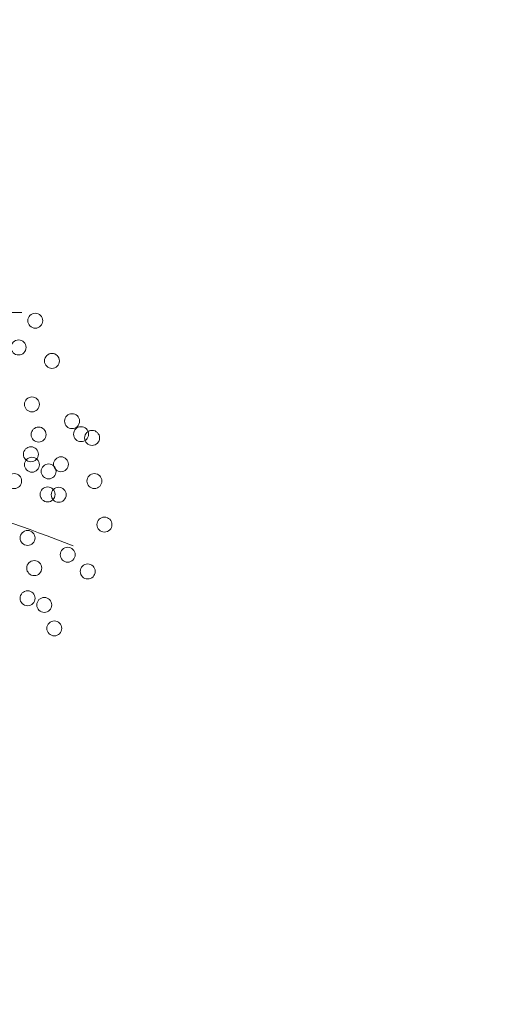
# Model space of a CAD drawing. Units: inches. Extents: x -48 to 50072, y 0 to 21068.
# Tile 8 of 75: x 233 to 245, y 253 to 278. Entities that reach past the tile are written whole.
import ezdxf

# ---------------------------------------------------------------- set-up
doc = ezdxf.new("R2010")
doc.units = ezdxf.units.IN
doc.header["$MEASUREMENT"] = 0
doc.layers.add('A-ANNO-DIMS', color=2, linetype='Continuous', lineweight=18)
doc.layers.add('L-PLNT', color=94, linetype='Continuous', lineweight=13)
doc.styles.get("Standard").update_dxf_attribs({"font": 'arial.ttf'})
doc.dimstyles.get("Standard").update_dxf_attribs({"dimtxt": 8, "dimasz": 0.18, "dimexe": 0.18, "dimexo": 0.0625, "dimgap": 0.09, "dimtad": 0, "dimtih": 1, "dimtoh": 1, "dimdec": 1, "dimzin": 0, "dimdsep": 46, "dimlunit": 4, "dimtxsty": 'Standard', "dimblk": 'ARCHTICK', "dimcen": 0.09, "dimadec": 0, "dimazin": 0, "dimtfac": 1, "dimtdec": 1, "dimtofl": 0, "dimtmove": 0, "dimatfit": 3, "dimldrblk": 'ARCHTICK', "dimfxl": 1, "dimtolj": 1, "dimtzin": 0, "dimarcsym": 0})

# ---------------------------------------------------------------- blocks, each defined once
blk = doc.blocks.new('A$C2ECE247B')
for centre in [(4.1847, 3.5734), (4.0942, 3.4285), (4.2753, 3.356), (4.1666, 3.1204), (4.3839, 3.0298), (4.2028, 2.9573), (4.4327, 2.9593), (4.4926, 2.9392), (4.161, 2.8505), (4.1666, 2.7943), (4.324, 2.7962), (4.2571, 2.758), (4.0705, 2.7056), (4.5051, 2.7056), (4.2516, 2.6331), (4.3115, 2.6312), (4.5594, 2.47), (4.1429, 2.3975), (4.3602, 2.3069), (4.1791, 2.2344), (4.4689, 2.2163), (4.1429, 2.0713), (4.2335, 2.0351), (4.2878, 1.9083)]:
    blk.add_circle(centre, 0.0405)
for points, knots in [([(2.2475, 2.6079), (2.3519, 2.8641), (2.6603, 3.6207), (3.5343, 3.6189), (4.1125, 3.6177)], [0, 0, 0, 0, 0.779419, 2.302165, 2.302165, 2.302165, 2.302165]), ([(3.18, 2.6079), (3.3323, 2.6059), (3.7494, 2.6004), (4.1411, 2.4506), (4.3897, 2.3554)], [0, 0, 0, 0, 0.454352, 1.243831, 1.243831, 1.243831, 1.243831])]:
    blk.add_open_spline(points, degree=3, knots=knots)
blk = doc.blocks.new('_ArchTick')
at = {"color": 0, "linetype": 'ByBlock', "const_width": 0.15}
blk.add_lwpolyline([(-0.5, -0.5), (0.5, 0.5)], dxfattribs=at)
blk = doc.blocks.new('*D52')
at = {"layer": 'A-ANNO-DIMS', "color": 0, "lineweight": -2, "transparency": 16777216}
for p, q in [((238.847, 252.654), (242.859, 252.654)), ((242.679, 252.654), (242.679, 243.897)), ((242.679, 226.686), (242.679, 235.444)), ((238.847, 226.686), (242.859, 226.686))]:
    blk.add_line(p, q, dxfattribs=at)
at = {"layer": 'Defpoints', "color": 0, "transparency": 16777216}
for p in [(238.784, 252.654), (242.679, 252.654), (238.784, 226.686)]:
    blk.add_point(p, dxfattribs=at)
at = {"layer": 'A-ANNO-DIMS', "color": 0, "lineweight": -2, "transparency": 16777216, "xscale": 0.18, "yscale": 0.18, "zscale": 0.18}
for p, rotation in [((242.679, 252.654), 90), ((242.679, 226.686), 270)]:
    blk.add_blockref('_ArchTick', p, dxfattribs=dict(at, rotation=rotation))
at = {"layer": 'A-ANNO-DIMS', "color": 0, "transparency": 16777216, "insert": (242.679, 239.67), "char_height": 8, "attachment_point": 5}
blk.add_mtext('\\A1;SHRUB A 26 TYP.', dxfattribs=at)
blk = doc.blocks.new('*D117')
at = {"layer": 'A-ANNO-DIMS', "color": 0, "lineweight": -2, "transparency": 16777216}
for p, q in [((216.017, 488.712), (216.017, 165.945)), ((297.017, 488.712), (297.017, 165.945)), ((216.017, 166.125), (251.464, 166.125)), ((297.017, 166.125), (261.57, 166.125))]:
    blk.add_line(p, q, dxfattribs=at)
at = {"layer": 'Defpoints', "color": 0, "transparency": 16777216}
for p in [(216.017, 488.775), (297.017, 488.775), (297.017, 166.125)]:
    blk.add_point(p, dxfattribs=at)
at = {"layer": 'A-ANNO-DIMS', "color": 0, "lineweight": -2, "transparency": 16777216, "xscale": 0.18, "yscale": 0.18, "zscale": 0.18, "rotation": 180}
blk.add_blockref('_ArchTick', (216.017, 166.125), dxfattribs=at)
at = {"layer": 'A-ANNO-DIMS', "color": 0, "lineweight": -2, "transparency": 16777216, "xscale": 0.18, "yscale": 0.18, "zscale": 0.18}
blk.add_blockref('_ArchTick', (297.017, 166.125), dxfattribs=at)
at = {"layer": 'A-ANNO-DIMS', "color": 0, "transparency": 16777216, "insert": (256.517, 166.125), "char_height": 8, "attachment_point": 5}
blk.add_mtext('\\A1;81', dxfattribs=at)

msp = doc.modelspace()

# ---------------------------------------------------------------- block references
at = {"layer": 'L-PLNT', "xscale": 4.644034438665709, "yscale": 4.644034438665709, "zscale": 4.644034438665709}
msp.add_blockref('A$C2ECE247B', (214.164, 253.826), dxfattribs=at)

# ---------------------------------------------------------------- dimensions: what is measured, and where the dimension line sits
at = {"layer": 'A-ANNO-DIMS'}
dim = msp.add_linear_dim(base=(297.017, 166.125), p1=(216.017, 488.775), p2=(297.017, 488.775), dimstyle='Standard', override={"dimdec": 0, "dimlfac": 1, "dimrnd": 0, "dimzin": 0, "dimdsep": 46, "dimlunit": 2}, dxfattribs=at)
dim.commit()
dim.dimension.update_dxf_attribs({"geometry": '*D117', "text_midpoint": (256.517, 166.125)})
dim = msp.add_linear_dim(base=(242.679, 252.654), p1=(238.784, 226.686), p2=(238.784, 252.654), angle=90, text='SHRUB A <> TYP.', dimstyle='Standard', override={"dimdec": 0, "dimlfac": 1, "dimrnd": 0, "dimzin": 0, "dimdsep": 46, "dimlunit": 2}, dxfattribs=at)
dim.commit()
dim.dimension.update_dxf_attribs({"geometry": '*D52', "text_midpoint": (242.679, 239.67)})

doc.saveas('drawing.dxf')
